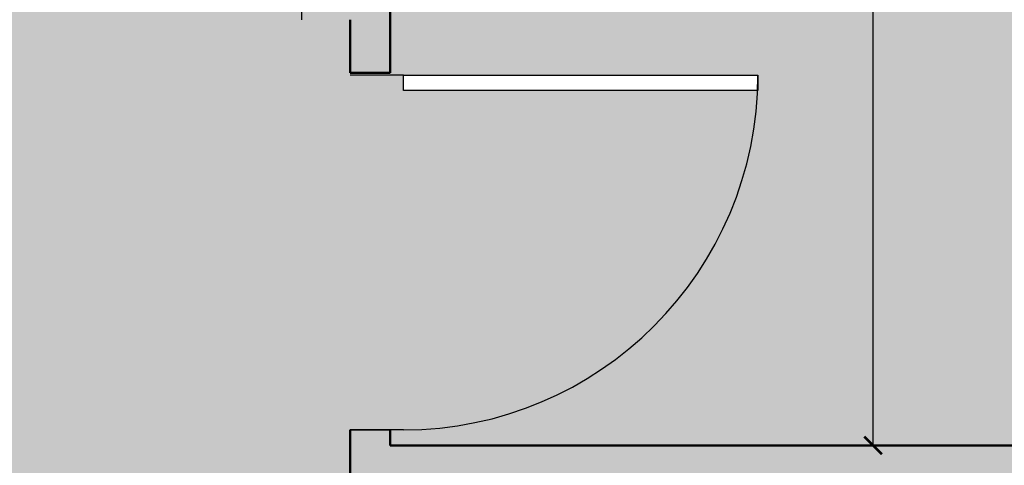
# Model space of a CAD drawing. Units: inches. Extents: x 528 to 2620, y -1066 to 798.
# Tile 10 of 41: x 737 to 848, y 523 to 573. Entities that reach past the tile are written whole.
import ezdxf

# ---------------------------------------------------------------- set-up
doc = ezdxf.new("R2010")
doc.units = ezdxf.units.IN
doc.header["$MEASUREMENT"] = 0
for name, color, linetype, lineweight in [('A-ANNO-DIMS', 2, 'Continuous', 18), ('A-Door', 2, 'Continuous', 25), ('A-WALL', 7, 'Continuous', 50), ('A-WALL-PATT', 8, 'Continuous', 13)]:
    doc.layers.add(name, color=color, linetype=linetype, lineweight=lineweight)
doc.styles.get("Standard").update_dxf_attribs({"font": 'arial.ttf'})
doc.dimstyles.get("Standard").update_dxf_attribs({"dimtxt": 6, "dimasz": 2, "dimexe": 0.18, "dimexo": 0.0625, "dimgap": 0.09, "dimtad": 0, "dimtih": 1, "dimtoh": 1, "dimdec": 1, "dimzin": 0, "dimdsep": 46, "dimlunit": 3, "dimtxsty": 'Standard', "dimblk": 'ARCHTICK', "dimcen": 0.09, "dimadec": 0, "dimazin": 0, "dimtfac": 1, "dimtdec": 1, "dimtofl": 0, "dimtmove": 0, "dimatfit": 3, "dimfxl": 1, "dimtolj": 1, "dimtzin": 0, "dimarcsym": 0})

# ---------------------------------------------------------------- blocks, each defined once
blk = doc.blocks.new('*U4')
for p, q in [((0, 0), (0, -6)), ((40, 0), (40, -6))]:
    blk.add_line(p, q)
blk.add_lwpolyline([(0, 0), (0, 40), (1.75, 40), (1.75, 0)], close=True)
blk.add_arc((0, 0), 40, 0, 90)
blk = doc.blocks.new('_ArchTick')
at = {"color": 0, "linetype": 'ByBlock', "const_width": 0.15}
blk.add_lwpolyline([(-0.5, -0.5), (0.5, 0.5)], dxfattribs=at)
blk = doc.blocks.new('*D28')
at = {"layer": 'A-ANNO-DIMS', "color": 0, "lineweight": -2, "transparency": 16777216}
for p, q in [((833.06, 709.92), (833.06, 620.83)), ((833.12, 709.92), (833.24, 709.92)), ((833.06, 525.42), (833.06, 614.52)), ((833.1, 525.42), (832.88, 525.42))]:
    blk.add_line(p, q, dxfattribs=at)
at = {"layer": 'Defpoints', "color": 0, "transparency": 16777216}
for p in [(833.06, 709.92), (833.06, 709.92), (833.16, 525.42)]:
    blk.add_point(p, dxfattribs=at)
at = {"layer": 'A-ANNO-DIMS', "color": 0, "lineweight": -2, "transparency": 16777216, "xscale": 2, "yscale": 2, "zscale": 2}
for p, rotation in [((833.06, 709.92), 90), ((833.06, 525.42), 270)]:
    blk.add_blockref('_ArchTick', p, dxfattribs=dict(at, rotation=rotation))
at = {"layer": 'A-ANNO-DIMS', "color": 0, "transparency": 16777216, "insert": (833.06, 617.67), "char_height": 6, "attachment_point": 5}
blk.add_mtext('\\A1;15\'-4.5"', dxfattribs=at)

msp = doc.modelspace()

# ---------------------------------------------------------------- hatches: boundary and pattern name
at = {"layer": 'A-WALL-PATT', "transparency": 33554521}
h = msp.add_hatch(color=256, dxfattribs=at)
h.dxf.hatch_style = 1
h.paths.add_polyline_path([(629.06, 709.92), (677.56, 709.92), (677.56, 718.92), (620.06, 718.92), (620.06, 667.92), (629.06, 667.92)])
h.paths.add_polyline_path([(790.56, 718.92), (725.56, 718.92), (725.56, 709.92), (774.06, 709.92), (774.06, 577.92), (768.48, 577.92), (768.56, 573.42), (774.06, 573.42), (774.06, 567.42), (778.56, 567.42), (778.56, 669.42), (831.06, 669.42), (831.06, 675.92), (826.56, 675.92), (826.56, 673.92), (778.56, 673.92), (778.56, 709.92), (790.56, 709.92)])
h.paths.add_polyline_path([(908.06, 718.92), (879.06, 718.92), (879.06, 709.92), (899.06, 709.92), (899.06, 641.67), (908.06, 641.67)])
h.paths.add_polyline_path([(629.06, 619.92), (620.06, 619.92), (620.06, 561.42), (629.06, 561.42), (629.06, 573.42), (724.06, 573.42), (724.06, 569.42), (728.56, 569.42), (728.56, 577.92), (629.06, 577.92)])
h.paths.add_polyline_path([(779.06, 391.42), (779.06, 400.42), (770.06, 400.42), (764.06, 400.42), (764.06, 397.42), (764.06, 391.42), (770.06, 391.42), (770.06, 268.92), (815.06, 268.92), (815.06, 277.92), (779.06, 277.92), (779.06, 359.77)])
h.paths.add_polyline_path([(908.06, 395.92), (899.06, 395.92), (851.06, 395.92), (851.06, 391.42), (899.06, 391.42), (899.06, 277.92), (863.06, 277.92), (863.06, 268.92), (908.06, 268.92)])
h.paths.add_polyline_path([(908.06, 593.67), (899.06, 593.67), (899.06, 525.42), (778.56, 525.42), (778.56, 527.17), (774.06, 527.17), (774.06, 520.92), (899.06, 520.92), (899.06, 443.92), (908.06, 443.92)])
h.paths.add_polyline_path([(629.06, 520.92), (728.56, 520.92), (728.56, 545.42), (724.06, 545.42), (724.06, 525.42), (629.06, 525.42), (629.06, 537.42), (620.06, 537.42), (620.06, 484.67), (629.06, 484.67)])
h.paths.add_polyline_path([(629.06, 436.67), (620.06, 436.67), (620.06, 391.42), (648.56, 391.42), (648.56, 400.42), (629.06, 400.42)])
h.paths.add_polyline_path([(716.06, 397.42), (716.06, 400.42), (696.56, 400.42), (696.56, 391.42), (716.06, 391.42)])
at = {"layer": 'A-WALL-PATT', "transparency": 33554590}
h = msp.add_hatch(color=256, dxfattribs=at)
h.dxf.hatch_style = 1
h.paths.add_polyline_path([(774.06, 709.92), (629.06, 709.92), (629.06, 577.92), (728.56, 577.92), (728.56, 579.42), (728.56, 619.42), (730.31, 619.42), (730.31, 619.38, -0.401453), (768.56, 579.42), (768.56, 577.92), (774.06, 577.92)])
h.paths.add_polyline_path([(723.9, 686.06), (723.97, 686.06), (723.83, 686.13)], flags=0)
h.paths.add_polyline_path([(722.79, 642.7), (722.89, 642.76), (722.89, 684.99), (722.65, 685.24), (722.65, 685.82), (723.08, 686.26), (723.53, 686.26), (723.97, 686.06), (724.74, 686.13), (770.7, 686.13), (770.78, 686.14), (771.13, 686.27), (771.69, 686.09), (771.94, 685.48), (771.67, 684.9), (771.58, 684.87), (771.58, 642.78), (771.88, 642.51), (771.88, 641.92), (771.51, 641.46), (770.85, 641.46), (770.4, 641.83), (770.4, 641.55), (724.74, 641.55), (723.99, 641.7), (723.44, 641.41), (722.88, 641.59), (722.6, 642.14)], flags=16)
h.paths.add_polyline_path([(723.99, 641.7), (723.99, 641.71), (723.99, 641.7)], flags=0)
h.paths.add_polyline_path([(722.89, 642.73), (722.89, 684.99), (722.65, 685.24), (722.65, 685.82), (723.08, 686.26), (723.29, 686.26), (722.99, 686.17), (722.79, 685.97), (722.65, 685.68), (722.65, 685.43), (722.75, 685.14), (722.94, 684.94), (723.24, 684.81), (723.48, 684.81), (723.78, 684.9), (723.98, 685.1), (724.17, 685.49), (724.12, 685.64), (724.12, 685.25), (723.63, 684.75), (723.63, 642.96), (724.12, 642.51), (724.12, 641.89), (723.66, 641.46), (723.08, 641.46), (722.65, 641.9), (722.65, 642.48)], flags=0)
h.paths.add_polyline_path([(722.65, 642.29), (722.65, 642.04), (722.79, 641.75), (723.08, 641.46), (723.29, 641.46), (722.88, 641.59), (722.6, 642.14)], flags=0)
h.paths.add_polyline_path([(770.75, 686.13), (770.58, 686.13), (770.55, 686.06)], flags=0)
h.paths.add_polyline_path([(743.3, 645.29), (753.23, 659.4), (748.69, 663.75), (753.23, 668.54), (743.3, 682.46), (743.79, 682.59), (744.14, 682.68), (744.53, 682.93), (744.63, 683.08), (745.02, 683.33), (744.53, 684.07), (744.78, 684.16), (744.87, 684.31), (745.51, 684.4), (746.08, 684.65), (746.47, 684.65), (746.82, 684.81), (747.46, 685.03), (747.71, 685.14), (748.2, 685.28), (748.39, 685.52), (748.86, 685.52), (749.99, 686.13), (753.49, 676.03), (757.38, 680.15), (757.79, 679.76), (758.04, 680.65), (758.29, 681.23), (758.29, 682.05), (758.02, 682.59), (757.87, 683.17), (757.82, 683.78), (758.39, 684.07), (758.98, 684.2), (759.62, 684.16), (760.21, 683.96), (760.75, 683.67), (761.86, 683.67), (762.4, 683.96), (762.99, 684.11), (763.63, 684.11), (764.2, 683.96), (764.74, 683.67), (766.12, 683.67), (766.66, 683.96), (767.25, 684.16), (767.87, 684.2), (768.46, 684.07), (769.05, 683.78), (769, 683.17), (768.85, 682.59), (768.55, 682.05), (768.55, 681.23), (768.8, 680.65), (769.09, 679.75), (768.95, 678.83), (768.8, 678.23), (768.55, 677.65), (768.55, 676.82), (768.8, 676.24), (769.09, 675.34), (768.95, 674.42), (768.8, 673.82), (768.55, 673.28), (768.55, 672.41), (768.8, 671.87), (769, 671.29), (769.05, 670.64), (768.95, 670.02), (768.8, 669.41), (768.55, 668.87), (768.55, 668), (768.97, 667.24), (769.05, 666.28), (769.05, 665.56), (768.46, 665.32), (767.87, 665.16), (767.25, 665.16), (766.66, 665.36), (766.12, 665.7), (764.74, 665.7), (763.94, 665.2), (762.99, 665.2), (762.4, 665.36), (761.86, 665.7), (761, 665.7), (762.7, 664.09), (760.74, 662.03), (761.86, 662.03), (762.4, 662.32), (763.34, 662.55), (764.25, 662.32), (764.79, 662.03), (766.12, 662.03), (766.66, 662.32), (767.25, 662.52), (767.87, 662.56), (768.51, 662.43), (769.05, 662.12), (769.05, 661.4), (769.05, 660.8), (768.85, 660.21), (768.55, 659.68), (768.55, 658.85), (768.85, 658.27), (769, 657.66), (769.07, 656.75), (768.85, 655.85), (768.55, 655.27), (768.55, 654.44), (768.85, 653.86), (769.07, 652.96), (769, 652.05), (768.85, 651.44), (768.55, 650.91), (768.55, 650.03), (768.85, 649.5), (769, 648.91), (769.05, 648.26), (769, 647.64), (768.85, 647.03), (768.55, 646.5), (768.55, 645.62), (768.85, 645.09), (769.05, 644.55), (769.05, 643.9), (768.51, 643.65), (767.87, 643.52), (767.25, 643.52), (766.66, 643.72), (766.12, 644.06), (764.79, 644.06), (764.25, 643.72), (763.34, 643.49), (762.4, 643.72), (761.86, 644.06), (760.8, 644.06), (760.26, 643.72), (759.67, 643.52), (759.03, 643.52), (758.39, 643.65), (757.87, 643.9), (757.87, 644.55), (758.04, 645.09), (758.34, 645.62), (758.34, 646.5), (758.04, 647.03), (757.92, 647.64), (757.87, 648.06), (757.38, 647.59), (753.42, 651.77), (749.99, 641.62), (749.5, 641.71), (749.35, 641.95), (748.54, 642.45), (747.31, 642.94), (746.65, 642.94), (746.33, 643.18), (745.51, 643.57), (744.53, 643.65), (745.01, 644.4), (744.63, 644.64), (744.14, 644.89), (743.79, 645.13)], flags=0)
h.paths.add_polyline_path([(755.66, 654.93), (756.54, 654.69), (757.53, 654.33), (756.64, 654.58)], flags=0)
h.paths.add_polyline_path([(758.34, 649.2), (758.34, 648.71), (758.59, 644.3), (758.59, 648.8)], flags=0)
h.paths.add_polyline_path([(758.34, 649.29), (758.09, 649.7), (758.36, 649.17)], flags=0)
h.paths.add_polyline_path([(755.66, 672.79), (756.49, 673.04), (757.36, 673.35), (757.35, 673.36), (756.64, 673.15)], flags=0)
h.paths.add_polyline_path([(760.26, 639.64), (771.41, 639.64), (771.41, 624.04), (760.26, 624.04)], flags=16)
h.paths.add_polyline_path([(761.38, 638.53), (770.29, 638.53), (770.29, 625.15), (761.38, 625.15)], flags=0)
edge = h.paths.add_edge_path(flags=0)
edge.add_ellipse((765.84, 631.84), major_axis=(-2.24, 2.24), ratio=1, start_angle=-45, end_angle=45, ccw=False)
edge.add_ellipse((765.84, 631.84), major_axis=(-2.24, 2.24), ratio=1, start_angle=-135, end_angle=-45, ccw=False)
edge.add_ellipse((765.84, 631.84), major_axis=(-2.24, 2.24), ratio=1, start_angle=135, end_angle=-135, ccw=False)
edge.add_ellipse((765.84, 631.84), major_axis=(-2.24, 2.24), ratio=1, start_angle=45, end_angle=135, ccw=False)
h.paths.add_polyline_path([(758.59, 683.42), (758.59, 678.92), (758.37, 678.58), (758.34, 678.43), (758.09, 678.05), (758.34, 678.52), (758.34, 679.01)], flags=0)
h.paths.add_polyline_path([(760.26, 688.04), (760.26, 703.64), (771.41, 703.64), (771.41, 688.04)], flags=16)
h.paths.add_polyline_path([(770.4, 685.39), (770.4, 685.85), (770.85, 686.22), (771.51, 686.22), (771.88, 685.76), (771.88, 685.17), (771.58, 684.9), (771.58, 642.78), (771.88, 642.51), (771.88, 641.92), (771.51, 641.46), (770.85, 641.46), (770.4, 641.83), (770.4, 642.29)], flags=0)
h.paths.add_polyline_path([(770.53, 642.68), (771.05, 643.01), (771.67, 642.77), (771.94, 642.2), (771.69, 641.59), (771.13, 641.41), (770.55, 641.62), (770.35, 642.13)], flags=16)
h.paths.add_polyline_path([(761.38, 689.15), (761.38, 702.53), (770.29, 702.53), (770.29, 689.15)], flags=0)
edge = h.paths.add_edge_path(flags=0)
edge.add_ellipse((765.84, 695.84), major_axis=(2.24, 2.24), ratio=1, start_angle=405, end_angle=495, ccw=False)
edge.add_ellipse((765.84, 695.84), major_axis=(2.24, 2.24), ratio=1, start_angle=675, end_angle=765, ccw=False)
edge.add_ellipse((765.84, 695.84), major_axis=(2.24, 2.24), ratio=1, start_angle=585, end_angle=675, ccw=False)
edge.add_ellipse((765.84, 695.84), major_axis=(2.24, 2.24), ratio=1, start_angle=495, end_angle=585, ccw=False)
h.paths.add_polyline_path([(770.7, 684.9), (770.94, 684.74), (771.41, 684.74), (771.73, 685.03), (771.88, 685.34), (771.88, 685.64), (771.69, 686.09), (771.58, 686.13), (771.88, 685.76), (771.88, 685.17), (771.41, 684.74), (770.85, 684.74)], flags=0)
h.paths.add_polyline_path([(899.06, 709.92), (831.06, 709.92), (831.06, 699.92), (829.81, 699.92), (829.81, 675.92), (831.06, 675.92), (831.06, 669.42), (778.56, 669.42), (778.56, 567.17), (780.06, 567.17), (820.06, 567.17), (820.06, 565.42), (820.02, 565.42, -0.401453), (780.06, 527.17), (778.56, 527.17), (778.56, 525.42), (899.06, 525.42)])
h.paths.add_polyline_path([(849.2, 636.01), (849.27, 636.02), (849.13, 636.08)], flags=0)
h.paths.add_polyline_path([(848.19, 634.95), (847.95, 635.2), (847.95, 635.78), (848.38, 636.22), (848.83, 636.22), (849.27, 636.02), (850.04, 636.08), (896, 636.08), (896.08, 636.1), (896.43, 636.22), (896.99, 636.05), (897.24, 635.43), (896.97, 634.86), (896.88, 634.83), (896.88, 592.74), (897.18, 592.47), (897.18, 591.88), (896.81, 591.42), (896.15, 591.42), (895.7, 591.79), (895.7, 591.51), (850.04, 591.51), (849.29, 591.66), (848.74, 591.37), (848.18, 591.54), (847.9, 592.1), (848.09, 592.65), (848.19, 592.71)], flags=16)
h.paths.add_polyline_path([(849.29, 591.66), (849.29, 591.66), (849.29, 591.66)], flags=16)
h.paths.add_polyline_path([(848.19, 634.95), (847.95, 635.2), (847.95, 635.78), (848.38, 636.22), (848.59, 636.22), (848.29, 636.13), (848.09, 635.93), (847.95, 635.64), (847.95, 635.39), (848.05, 635.1), (848.24, 634.9), (848.54, 634.76), (848.78, 634.76), (849.08, 634.85), (849.28, 635.05), (849.47, 635.44), (849.42, 635.59), (849.42, 635.21), (848.93, 634.7), (848.93, 592.92), (849.42, 592.47), (849.42, 591.84), (848.96, 591.42), (848.38, 591.42), (847.95, 591.86), (847.95, 592.44), (848.19, 592.69)], flags=0)
h.paths.add_polyline_path([(847.95, 592.25), (847.95, 592), (848.09, 591.71), (848.38, 591.42), (848.59, 591.42), (848.18, 591.54), (847.9, 592.1)], flags=16)
h.paths.add_polyline_path([(896.05, 636.08), (895.88, 636.08), (895.85, 636.01)], flags=0)
h.paths.add_polyline_path([(868.6, 632.41), (869.09, 632.55), (869.44, 632.64), (869.83, 632.88), (869.93, 633.04), (870.32, 633.28), (869.83, 634.02), (870.08, 634.11), (870.17, 634.27), (870.81, 634.36), (871.38, 634.61), (871.77, 634.61), (872.12, 634.76), (872.76, 634.99), (873.01, 635.1), (873.5, 635.23), (873.69, 635.48), (874.16, 635.48), (875.29, 636.08), (878.79, 625.99), (882.68, 630.11), (883.09, 629.71), (883.34, 630.6), (883.59, 631.18), (883.59, 632.01), (883.32, 632.55), (883.17, 633.13), (883.12, 633.73), (883.69, 634.02), (884.28, 634.16), (884.92, 634.11), (885.51, 633.91), (886.05, 633.62), (887.16, 633.62), (887.7, 633.91), (888.29, 634.07), (888.93, 634.07), (889.5, 633.91), (890.04, 633.62), (891.42, 633.62), (891.96, 633.91), (892.55, 634.11), (893.17, 634.16), (893.76, 634.02), (894.35, 633.73), (894.3, 633.13), (894.15, 632.55), (893.85, 632.01), (893.85, 631.18), (894.1, 630.6), (894.39, 629.71), (894.25, 628.79), (894.1, 628.18), (893.85, 627.6), (893.85, 626.77), (894.1, 626.19), (894.39, 625.3), (894.25, 624.38), (894.1, 623.78), (893.85, 623.24), (893.85, 622.37), (894.1, 621.83), (894.3, 621.25), (894.35, 620.6), (894.25, 619.97), (894.1, 619.37), (893.85, 618.83), (893.85, 617.96), (894.27, 617.2), (894.35, 616.23), (894.35, 615.52), (893.76, 615.27), (893.17, 615.12), (892.55, 615.12), (891.96, 615.32), (891.42, 615.65), (890.04, 615.65), (889.25, 615.16), (888.29, 615.16), (887.7, 615.32), (887.16, 615.65), (886.31, 615.65), (888, 614.04), (886.04, 611.98), (887.16, 611.98), (887.7, 612.27), (888.64, 612.5), (889.55, 612.27), (890.09, 611.98), (891.42, 611.98), (891.96, 612.27), (892.55, 612.48), (893.17, 612.52), (893.81, 612.39), (894.35, 612.07), (894.35, 611.36), (894.35, 610.75), (894.15, 610.17), (893.85, 609.63), (893.85, 608.81), (894.15, 608.22), (894.3, 607.62), (894.37, 606.7), (894.15, 605.81), (893.85, 605.22), (893.85, 604.4), (894.15, 603.81), (894.37, 602.92), (894.3, 602), (894.15, 601.4), (893.85, 600.86), (893.85, 599.99), (894.15, 599.45), (894.3, 598.87), (894.35, 598.22), (894.3, 597.59), (894.15, 596.99), (893.85, 596.45), (893.85, 595.58), (894.15, 595.04), (894.35, 594.51), (894.35, 593.86), (893.81, 593.61), (893.17, 593.48), (892.55, 593.48), (891.96, 593.68), (891.42, 594.01), (890.09, 594.01), (889.55, 593.68), (888.64, 593.45), (887.7, 593.68), (887.16, 594.01), (886.1, 594.01), (885.56, 593.68), (884.97, 593.48), (884.33, 593.48), (883.69, 593.61), (883.17, 593.86), (883.17, 594.51), (883.34, 595.04), (883.64, 595.58), (883.64, 596.45), (883.34, 596.99), (883.22, 597.59), (883.17, 598.01), (882.68, 597.55), (878.72, 601.73), (875.29, 591.57), (874.8, 591.66), (874.65, 591.91), (873.84, 592.4), (872.61, 592.89), (871.95, 592.89), (871.63, 593.14), (870.81, 593.52), (869.83, 593.61), (870.31, 594.36), (869.93, 594.6), (869.44, 594.84), (869.09, 595.09), (868.6, 595.24), (878.53, 609.35), (873.99, 613.71), (878.53, 618.49)], flags=0)
h.paths.add_polyline_path([(880.96, 622.75), (881.79, 622.99), (882.66, 623.31), (882.65, 623.31), (881.94, 623.1)], flags=0)
h.paths.add_polyline_path([(880.96, 604.89), (881.84, 604.64), (882.83, 604.28), (881.94, 604.53)], flags=16)
h.paths.add_polyline_path([(883.39, 628.01), (883.64, 628.48), (883.64, 628.97), (883.89, 633.38), (883.89, 628.88), (883.67, 628.53), (883.64, 628.39)], flags=0)
h.paths.add_polyline_path([(883.64, 599.16), (883.64, 598.67), (883.89, 594.26), (883.89, 598.76)], flags=16)
h.paths.add_polyline_path([(883.64, 599.25), (883.39, 599.65), (883.66, 599.12)], flags=16)
h.paths.add_polyline_path([(885.56, 637.99), (885.56, 653.6), (896.71, 653.6), (896.71, 637.99)], flags=16)
h.paths.add_polyline_path([(885.56, 589.6), (896.71, 589.6), (896.71, 573.99), (885.56, 573.99)], flags=16)
h.paths.add_polyline_path([(886.68, 639.11), (886.68, 652.48), (895.59, 652.48), (895.59, 639.11)], flags=0)
h.paths.add_polyline_path([(886.68, 588.48), (895.59, 588.48), (895.59, 575.11), (886.68, 575.11)], flags=0)
edge = h.paths.add_edge_path(flags=0)
edge.add_ellipse((891.14, 645.79), major_axis=(2.24, 2.24), ratio=1, start_angle=405, end_angle=495, ccw=False)
edge.add_ellipse((891.14, 645.79), major_axis=(2.24, 2.24), ratio=1, start_angle=675, end_angle=765, ccw=False)
edge.add_ellipse((891.14, 645.79), major_axis=(2.24, 2.24), ratio=1, start_angle=585, end_angle=675, ccw=False)
edge.add_ellipse((891.14, 645.79), major_axis=(2.24, 2.24), ratio=1, start_angle=495, end_angle=585, ccw=False)
edge = h.paths.add_edge_path(flags=0)
edge.add_ellipse((891.14, 581.8), major_axis=(-2.24, 2.24), ratio=1, start_angle=-45, end_angle=45, ccw=False)
edge.add_ellipse((891.14, 581.8), major_axis=(-2.24, 2.24), ratio=1, start_angle=-135, end_angle=-45, ccw=False)
edge.add_ellipse((891.14, 581.8), major_axis=(-2.24, 2.24), ratio=1, start_angle=135, end_angle=-135, ccw=False)
edge.add_ellipse((891.14, 581.8), major_axis=(-2.24, 2.24), ratio=1, start_angle=45, end_angle=135, ccw=False)
h.paths.add_polyline_path([(895.7, 635.35), (895.7, 635.8), (896.15, 636.17), (896.81, 636.17), (897.18, 635.71), (897.18, 635.12), (896.88, 634.85), (896.88, 592.74), (897.18, 592.47), (897.18, 591.88), (896.81, 591.42), (896.15, 591.42), (895.7, 591.79), (895.7, 592.25)], flags=0)
h.paths.add_polyline_path([(896, 634.85), (896.24, 634.7), (896.71, 634.7), (897.03, 634.99), (897.18, 635.3), (897.18, 635.59), (896.99, 636.05), (896.88, 636.08), (897.18, 635.71), (897.18, 635.12), (896.71, 634.7), (896.15, 634.7)], flags=0)
h.paths.add_polyline_path([(895.83, 592.63), (896.35, 592.96), (896.97, 592.73), (897.24, 592.16), (896.99, 591.54), (896.43, 591.37), (895.85, 591.58), (895.65, 592.09)], flags=16)
h.paths.add_polyline_path([(725.25, 569.42), (724.06, 569.42), (724.06, 573.42), (629.06, 573.42), (629.06, 525.42), (724.06, 525.42), (724.06, 545.42), (725.25, 545.42)])
h.paths.add_polyline_path([(820.02, 565.42), (780.06, 565.42), (780.06, 567.17), (774.06, 567.17), (774.06, 567.42), (774.06, 573.42), (768.56, 573.42), (768.48, 577.92), (768.56, 577.92), (768.56, 579.42, 0.401453), (730.31, 619.38), (730.31, 579.42), (728.56, 579.42), (728.56, 573.42), (728.56, 569.42), (727.25, 569.42), (727.25, 545.42), (728.56, 545.42), (728.56, 520.92), (665.06, 520.92), (665.06, 436.42), (716.06, 436.42), (716.06, 421.42), (717.81, 421.42), (717.81, 421.36, -0.392996), (740.06, 397.42, -0.392996), (762.31, 421.36), (762.31, 421.42), (764.06, 421.42), (764.06, 400.42), (770.06, 400.42), (779.06, 400.42), (779.06, 391.42), (779.06, 359.77), (795.43, 359.77), (795.43, 294.3), (893.67, 294.3), (893.67, 277.92), (899.06, 277.92), (899.06, 391.42), (851.06, 391.42), (851.06, 395.92), (899.06, 395.92), (899.06, 443.92), (899.06, 520.92), (774.06, 520.92), (774.06, 527.17), (778.56, 527.17), (780.06, 527.17, 0.401453)])
h.paths.add_polyline_path([(774.06, 519.66), (842.12, 519.66), (842.12, 505.07), (788.64, 505.07), (788.64, 474.08), (788.64, 470.43, -0.883215), (779.53, 456.66), (774.97, 456.66, -0.414214), (774.06, 457.57)], flags=16)
h.paths.add_polyline_path([(775.88, 517.83), (840.3, 517.83), (840.3, 514.19), (788.64, 514.19), (788.64, 484.41), (779.53, 484.41), (779.53, 474.08), (775.88, 474.08)], flags=0)
h.paths.add_polyline_path([(706.7, 501.56, -0.254069), (706.7, 493.02), (698.31, 492.55), (698.31, 502.03)], flags=16)
h.paths.add_polyline_path([(691.33, 515.69), (691.8, 507.3), (682.32, 507.3), (682.79, 515.69, -0.254069)], flags=16)
h.paths.add_polyline_path([(695.49, 504.68), (695.49, 479.42), (678.64, 479.42), (678.64, 504.68)], flags=16)
h.paths.add_polyline_path([(706.7, 489.6, -0.254069), (706.7, 481.06), (698.31, 480.59), (698.31, 490.07)], flags=16)
h.paths.add_polyline_path([(675.81, 502.03), (675.81, 492.55), (667.42, 493.02, -0.254069), (667.42, 501.56)], flags=16)
h.paths.add_polyline_path([(691.8, 476.8), (691.33, 468.41, -0.254069), (682.79, 468.41), (682.32, 476.8)], flags=16)
h.paths.add_polyline_path([(675.81, 490.07), (675.81, 480.59), (667.42, 481.06, -0.254069), (667.42, 489.6)], flags=16)
h.paths.add_polyline_path([(764.06, 397.42), (762.31, 397.42), (762.31, 421.36, 0.392996), (740.06, 397.42, 0.392996), (717.81, 421.36), (717.81, 397.42), (716.06, 397.42), (716.06, 391.42), (716.06, 385.42), (764.06, 385.42), (764.06, 391.42)], flags=17)
h.paths.add_polyline_path([(716.06, 436.42), (705.86, 436.42), (705.86, 418.42), (716.06, 418.42), (716.06, 421.42)], flags=17)
h.paths.add_polyline_path([(716.06, 418.42), (705.86, 418.42), (705.86, 400.42), (716.06, 400.42)], flags=17)
h.paths.add_polyline_path([(705.86, 418.42), (695.66, 418.42), (695.66, 400.42), (696.56, 400.42), (705.86, 400.42)], flags=17)
h.paths.add_polyline_path([(705.86, 436.42), (695.66, 436.42), (695.66, 418.42), (705.86, 418.42)], flags=17)
h.paths.add_polyline_path([(695.66, 418.42), (685.46, 418.42), (685.46, 400.42), (695.66, 400.42)], flags=17)
h.paths.add_polyline_path([(695.66, 436.42), (685.46, 436.42), (685.46, 418.42), (695.66, 418.42)], flags=17)
h.paths.add_polyline_path([(685.46, 418.42), (675.26, 418.42), (675.26, 400.42), (685.46, 400.42)], flags=17)
h.paths.add_polyline_path([(685.46, 436.42), (675.26, 436.42), (675.26, 418.42), (685.46, 418.42)], flags=17)
h.paths.add_polyline_path([(675.26, 436.42), (665.06, 436.42), (665.06, 418.42), (675.26, 418.42)])
h.paths.add_polyline_path([(675.26, 418.42), (665.06, 418.42), (665.06, 400.42), (675.26, 400.42)])
h.paths.add_polyline_path([(665.06, 418.42), (646.97, 418.42), (646.99, 436.42), (629.06, 436.42), (629.06, 400.42), (665.06, 400.42)])
h.paths.add_polyline_path([(665.06, 436.42), (646.99, 436.42), (646.97, 418.42), (665.06, 418.42)], flags=17)
h.paths.add_polyline_path([(647.01, 446.62), (629.06, 446.62), (629.06, 436.67), (629.06, 436.42), (646.99, 436.42)])
h.paths.add_polyline_path([(665.06, 446.62), (647.01, 446.62), (646.99, 436.42), (665.06, 436.42)])
h.paths.add_polyline_path([(647.02, 456.82), (629.06, 456.82), (629.06, 446.62), (647.01, 446.62)])
h.paths.add_polyline_path([(665.06, 456.82), (647.02, 456.82), (647.01, 446.62), (665.06, 446.62)])
h.paths.add_polyline_path([(647.03, 467.02), (629.06, 467.02), (629.06, 456.82), (647.02, 456.82)])
h.paths.add_polyline_path([(665.06, 467.02), (647.03, 467.02), (647.02, 456.82), (665.06, 456.82)])
h.paths.add_polyline_path([(665.06, 477.22), (647.05, 477.22), (647.03, 467.02), (665.06, 467.02)])
h.paths.add_polyline_path([(647.05, 477.22), (629.06, 477.22), (629.06, 467.02), (647.03, 467.02)])
h.paths.add_polyline_path([(647.06, 487.22), (629.06, 487.22), (629.06, 477.22), (647.05, 477.22), (647.05, 479.02), (645.53, 483.25), (640.88, 480.37)])
h.paths.add_polyline_path([(665.06, 520.92), (629.06, 520.92), (629.06, 487.22), (647.06, 487.22), (665.06, 487.22)])
h.paths.add_polyline_path([(665.06, 487.22), (647.06, 487.22), (653.22, 480.35), (648.58, 483.24), (647.05, 479.02), (647.05, 477.22), (665.06, 477.22)])

# ---------------------------------------------------------------- linework, layer by layer
at = {"layer": 'A-Door'}
msp.add_line((774.06, 527.17), (778.56, 527.17), dxfattribs=at)
at = {"layer": 'A-WALL'}
for p, q in [((778.56, 669.42), (778.56, 567.42)), ((774.06, 573.42), (774.06, 567.42)), ((774.06, 567.42), (778.56, 567.42)), ((774.06, 527.17), (774.06, 520.92)), ((778.56, 527.17), (778.56, 525.42)), ((899.06, 525.42), (778.56, 525.42))]:
    msp.add_line(p, q, dxfattribs=at)

# ---------------------------------------------------------------- block references
at = {"layer": 'A-Door'}
msp.add_blockref('*U4', (728.56, 579.42), dxfattribs=at)
at = {"layer": 'A-Door', "rotation": 270}
msp.add_blockref('*U4', (780.06, 567.17), dxfattribs=at)

# ---------------------------------------------------------------- dimensions: what is measured, and where the dimension line sits
at = {"layer": 'A-ANNO-DIMS'}
dim = msp.add_linear_dim(base=(833.06, 709.92), p1=(833.16, 525.42), p2=(833.06, 709.92), angle=90, dimstyle='Standard', override={"dimclrd": 0, "dimclre": 0, "dimclrt": 0}, dxfattribs=at)
dim.commit()
dim.dimension.update_dxf_attribs({"geometry": '*D28', "text_midpoint": (833.06, 617.67)})

doc.saveas('drawing.dxf')
